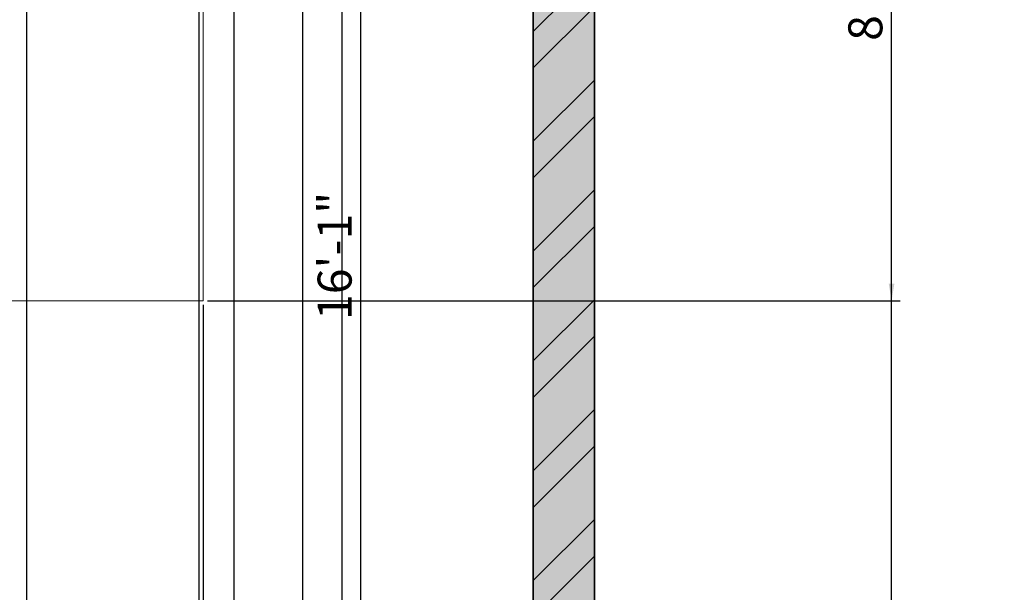
# Model space of a CAD drawing. Units: inches. Extents: x 1804 to 3296, y 909 to 2477.
# Tile 20 of 31: x 2241 to 2386, y 1638 to 1722. Entities that reach past the tile are written whole.
import ezdxf

# ---------------------------------------------------------------- set-up
doc = ezdxf.new("R2010")
doc.units = ezdxf.units.IN
for name, color, linetype, lineweight in [('A-ANNO-DIMS', 2, 'Continuous', 18), ('A-ANNO-TTLB', 156, 'Continuous', 35), ('A-WALL-PATT', 10, 'Continuous', 13), ('FUR', 100, 'Continuous', 18), ('WALL', 10, 'Continuous', 35)]:
    doc.layers.add(name, color=color, linetype=linetype, lineweight=lineweight)
doc.styles.get("Standard").update_dxf_attribs({"font": 'arial.ttf'})
doc.dimstyles.new('ISO-25', dxfattribs={"dimtxt": 5, "dimasz": 2.5, "dimexe": 1.25, "dimexo": 0.625, "dimtad": 1, "dimdec": 0, "dimlunit": 4, "dimtxsty": 'Standard', "dimcen": 2.5, "dimadec": 0, "dimazin": 0, "dimtfac": 1, "dimtdec": 0, "dimtmove": 0, "dimatfit": 3, "dimfxl": 1, "dimarcsym": 0})

# ---------------------------------------------------------------- blocks, each defined once
blk = doc.blocks.new('*D11')
at = {"layer": 'A-ANNO-DIMS', "color": 0, "lineweight": -2, "transparency": 16777216}
for p, q in [((2315.91, 1784.38), (2289.92, 1784.38)), ((2291.17, 1781.88), (2291.17, 1593.42)), ((2315.91, 1590.92), (2289.92, 1590.92))]:
    blk.add_line(p, q, dxfattribs=at)
at = {"layer": 'A-ANNO-DIMS', "color": 0, "lineweight": 100, "transparency": 16777216}
for points in [[(2290.75, 1781.88), (2291.58, 1781.88), (2291.17, 1784.38)], [(2290.75, 1593.42), (2291.58, 1593.42), (2291.17, 1590.92)]]:
    blk.add_solid(points, dxfattribs=at)
at = {"layer": 'Defpoints', "color": 0, "lineweight": 100, "transparency": 16777216}
for p in [(2316.54, 1784.38), (2291.17, 1590.92), (2316.54, 1590.92)]:
    blk.add_point(p, dxfattribs=at)
at = {"layer": 'A-ANNO-DIMS', "color": 0, "transparency": 16777216, "insert": (2287.99, 1687.65), "char_height": 5, "attachment_point": 5, "rotation": 90}
blk.add_mtext('16\'-1"', dxfattribs=at)
blk = doc.blocks.new('*D53')
at = {"layer": 'A-ANNO-DIMS', "color": 0, "lineweight": -2, "transparency": 16777216}
for p, q in [((2326.16, 1793.38), (2370.49, 1793.38)), ((2369.24, 1140.57), (2369.24, 1790.88)), ((2326.16, 1138.07), (2370.49, 1138.07))]:
    blk.add_line(p, q, dxfattribs=at)
at = {"layer": 'A-ANNO-DIMS', "color": 0, "lineweight": 100, "transparency": 16777216}
for points in [[(2368.82, 1790.88), (2369.65, 1790.88), (2369.24, 1793.38)], [(2368.82, 1140.57), (2369.65, 1140.57), (2369.24, 1138.07)]]:
    blk.add_solid(points, dxfattribs=at)
at = {"layer": 'Defpoints', "color": 0, "lineweight": 100, "transparency": 16777216}
for p in [(2325.54, 1793.38), (2369.24, 1793.38), (2325.54, 1138.07)]:
    blk.add_point(p, dxfattribs=at)
at = {"layer": 'A-ANNO-DIMS', "color": 0, "transparency": 16777216, "insert": (2366.03, 1465.72), "char_height": 5, "attachment_point": 5, "rotation": 90}
blk.add_mtext('54\'-7 1/2"', dxfattribs=at)
blk = doc.blocks.new('*D56')
at = {"layer": 'A-ANNO-DIMS', "color": 0, "lineweight": -2, "transparency": 16777216}
for p, q in [((2180.87, 1680.42), (2180.87, 975.89)), ((2268, 1680.42), (2268, 975.89)), ((2183.37, 977.14), (2265.5, 977.14))]:
    blk.add_line(p, q, dxfattribs=at)
at = {"layer": 'A-ANNO-DIMS', "color": 0, "lineweight": 100, "transparency": 16777216}
for points in [[(2183.37, 977.56), (2183.37, 976.72), (2180.87, 977.14)], [(2265.5, 977.56), (2265.5, 976.72), (2268, 977.14)]]:
    blk.add_solid(points, dxfattribs=at)
at = {"layer": 'Defpoints', "color": 0, "lineweight": 100, "transparency": 16777216}
for p in [(2180.87, 1681.04), (2268, 1681.04), (2268, 977.14)]:
    blk.add_point(p, dxfattribs=at)
at = {"layer": 'A-ANNO-DIMS', "color": 0, "transparency": 16777216, "insert": (2224.44, 980.32), "char_height": 5, "attachment_point": 5}
blk.add_mtext('7\'-3"', dxfattribs=at)
blk = doc.blocks.new('*D57')
at = {"layer": 'A-ANNO-DIMS', "color": 0, "lineweight": -2, "transparency": 16777216}
for p, q in [((2268.63, 1784.38), (2370.49, 1784.38)), ((2369.24, 1683.54), (2369.24, 1781.88)), ((2268.63, 1681.04), (2370.49, 1681.04))]:
    blk.add_line(p, q, dxfattribs=at)
at = {"layer": 'A-ANNO-DIMS', "color": 0, "lineweight": 100, "transparency": 16777216}
for points in [[(2368.82, 1781.88), (2369.65, 1781.88), (2369.24, 1784.38)], [(2368.82, 1683.54), (2369.65, 1683.54), (2369.24, 1681.04)]]:
    blk.add_solid(points, dxfattribs=at)
at = {"layer": 'Defpoints', "color": 0, "lineweight": 100, "transparency": 16777216}
for p in [(2268, 1784.38), (2369.24, 1784.38), (2268, 1681.04)]:
    blk.add_point(p, dxfattribs=at)
at = {"layer": 'A-ANNO-DIMS', "color": 0, "transparency": 16777216, "insert": (2366.03, 1732.71), "char_height": 5, "attachment_point": 5, "rotation": 90}
blk.add_mtext('8\'-7 1/2"', dxfattribs=at)
blk = doc.blocks.new('*D65')
at = {"layer": 'A-ANNO-DIMS', "color": 0, "lineweight": -2, "transparency": 16777216}
for p, q in [((2282.65, 1466.57), (2282.65, 1874.99)), ((2316.54, 1466.57), (2316.54, 1874.99)), ((2285.15, 1873.74), (2314.04, 1873.74))]:
    blk.add_line(p, q, dxfattribs=at)
at = {"layer": 'A-ANNO-DIMS', "color": 0, "lineweight": 100, "transparency": 16777216}
for points in [[(2285.15, 1874.15), (2285.15, 1873.32), (2282.65, 1873.74)], [(2314.04, 1874.15), (2314.04, 1873.32), (2316.54, 1873.74)]]:
    blk.add_solid(points, dxfattribs=at)
at = {"layer": 'Defpoints', "color": 0, "lineweight": 100, "transparency": 16777216}
for p in [(2316.54, 1873.74), (2282.65, 1465.94), (2316.54, 1465.94)]:
    blk.add_point(p, dxfattribs=at)
at = {"layer": 'A-ANNO-DIMS', "color": 0, "transparency": 16777216, "insert": (2299.6, 1876.91), "char_height": 5, "attachment_point": 5}
blk.add_mtext('2\'-10"', dxfattribs=at)
blk = doc.blocks.new('*D67')
at = {"layer": 'A-ANNO-DIMS', "color": 0, "lineweight": -2, "transparency": 16777216}
for p, q in [((2267.43, 1587.05), (2267.43, 1874.99)), ((2288.43, 1587.05), (2288.43, 1874.99)), ((2269.93, 1873.74), (2285.93, 1873.74))]:
    blk.add_line(p, q, dxfattribs=at)
at = {"layer": 'A-ANNO-DIMS', "color": 0, "lineweight": 100, "transparency": 16777216}
for points in [[(2269.93, 1874.15), (2269.93, 1873.32), (2267.43, 1873.74)], [(2285.93, 1874.15), (2285.93, 1873.32), (2288.43, 1873.74)]]:
    blk.add_solid(points, dxfattribs=at)
at = {"layer": 'Defpoints', "color": 0, "lineweight": 100, "transparency": 16777216}
for p in [(2288.43, 1873.74), (2267.43, 1586.42), (2288.43, 1586.42)]:
    blk.add_point(p, dxfattribs=at)
at = {"layer": 'A-ANNO-DIMS', "color": 0, "transparency": 16777216, "insert": (2277.93, 1876.91), "char_height": 5, "attachment_point": 5}
blk.add_mtext('1\'-9"', dxfattribs=at)
blk = doc.blocks.new('*D68')
at = {"layer": 'A-ANNO-DIMS', "color": 0, "lineweight": -2, "transparency": 16777216}
for p, q in [((2242.06, 1587.05), (2242.06, 1874.99)), ((2267.43, 1587.05), (2267.43, 1874.99)), ((2244.56, 1873.74), (2264.93, 1873.74)), ((2267.43, 1873.74), (2296.2, 1873.74))]:
    blk.add_line(p, q, dxfattribs=at)
at = {"layer": 'A-ANNO-DIMS', "color": 0, "lineweight": 100, "transparency": 16777216}
for points in [[(2244.56, 1874.15), (2244.56, 1873.32), (2242.06, 1873.74)], [(2264.93, 1874.15), (2264.93, 1873.32), (2267.43, 1873.74)]]:
    blk.add_solid(points, dxfattribs=at)
at = {"layer": 'Defpoints', "color": 0, "lineweight": 100, "transparency": 16777216}
for p in [(2267.43, 1873.74), (2242.06, 1586.42), (2267.43, 1586.42)]:
    blk.add_point(p, dxfattribs=at)
at = {"layer": 'A-ANNO-DIMS', "color": 0, "transparency": 16777216, "insert": (2283.07, 1876.95), "char_height": 5, "attachment_point": 5}
blk.add_mtext('2\'-1 1/2"', dxfattribs=at)
blk = doc.blocks.new('*D73')
at = {"layer": 'A-ANNO-DIMS', "color": 0, "lineweight": -2, "transparency": 16777216}
for p, q in [((2272.59, 1272.26), (2272.59, 1874.99)), ((2316.54, 1272.26), (2316.54, 1874.99)), ((2275.09, 1873.74), (2314.04, 1873.74))]:
    blk.add_line(p, q, dxfattribs=at)
at = {"layer": 'A-ANNO-DIMS', "color": 0, "lineweight": 100, "transparency": 16777216}
for points in [[(2275.09, 1874.15), (2275.09, 1873.32), (2272.59, 1873.74)], [(2314.04, 1874.15), (2314.04, 1873.32), (2316.54, 1873.74)]]:
    blk.add_solid(points, dxfattribs=at)
at = {"layer": 'Defpoints', "color": 0, "lineweight": 100, "transparency": 16777216}
for p in [(2316.54, 1873.74), (2272.59, 1271.63), (2316.54, 1271.63)]:
    blk.add_point(p, dxfattribs=at)
at = {"layer": 'A-ANNO-DIMS', "color": 0, "transparency": 16777216, "insert": (2294.56, 1876.92), "char_height": 5, "attachment_point": 5}
blk.add_mtext('3\'-8"', dxfattribs=at)

msp = doc.modelspace()

# ---------------------------------------------------------------- hatches: boundary and pattern name
at = {"layer": 'A-ANNO-TTLB'}
h = msp.add_hatch(color=256, dxfattribs=at)
h.dxf.hatch_style = 1
h.paths.add_polyline_path([(3294.53, 2476.54), (1803.79, 2476.54), (1805.43, 909.47), (3296.17, 909.47)])
h.paths.add_polyline_path([(1811, 914.33), (1812.79, 2467.54), (3285.53, 2467.54), (3283.74, 914.33)], flags=16)
h.paths.add_polyline_path([(1925.58, 1062.77), (1925.58, 1138.07), (1925.58, 1539.88), (1925.58, 1793.38), (1925.58, 1830.04), (2325.54, 1830.04), (2325.54, 1793.38), (2325.54, 1586.42), (2325.54, 1138.07), (2325.54, 1062.77)], flags=0)
h.paths.add_polyline_path([(1997.22, 1029.4), (2008.85, 1037.96), (2008.85, 1020.84)], flags=0)
h.paths.add_polyline_path([(1934.58, 1138.07), (1934.58, 1147.07), (2078.77, 1147.07), (2078.77, 1138.07), (2060.94, 1138.07)], flags=0)
h.paths.add_polyline_path([(1944.35, 1138.07), (1944.35, 1147.07), (2056.05, 1147.07), (2056.05, 1138.07)], flags=0)
h.paths.add_polyline_path([(2222.24, 1037.96), (2233.87, 1029.4), (2222.24, 1020.84)], flags=0)
h.paths.add_polyline_path([(2061.94, 1139.07), (2061.94, 1146.07), (2077.77, 1146.07), (2077.77, 1139.07)], flags=0)
h.paths.add_polyline_path([(2149.58, 1138.07), (2149.58, 1269.44), (2158.58, 1269.44), (2158.58, 1326.69), (2149.58, 1326.69), (2149.58, 1340.94), (2139.6, 1340.94), (2139.6, 1434.25), (2149.58, 1434.25), (2149.58, 1447.36), (2158.58, 1447.36), (2158.58, 1423.87), (2158.58, 1408.06), (2198.46, 1408.06), (2198.46, 1412.56), (2282.65, 1412.56), (2282.65, 1465.94), (2316.54, 1465.94), (2316.54, 1590.92), (2192.86, 1590.92), (2192.86, 1595.3), (2291.17, 1595.3), (2291.17, 1590.92), (2316.54, 1590.92), (2316.54, 1784.38), (2300.24, 1784.38), (2300.24, 1757.47), (2268, 1757.47), (2268, 1681.04), (2180.87, 1681.04), (2180.87, 1757.47), (2148.63, 1757.47), (2148.63, 1784.38), (2119.08, 1784.38), (2119.08, 1585.58), (2114.58, 1585.58), (2114.58, 1784.38), (2064.11, 1784.38), (2046.28, 1784.38), (2046.28, 1760.38), (1958.58, 1760.38), (1958.58, 1664.38), (1934.58, 1664.38), (1934.58, 1784.38), (1934.58, 1793.38), (2046.28, 1793.38), (2064.11, 1793.38), (2119.08, 1793.38), (2230.78, 1793.38), (2230.78, 1784.38), (2268, 1784.38), (2300.24, 1784.38), (2316.54, 1784.38), (2316.54, 1590.92), (2316.54, 1373.73), (2316.54, 1138.07)], flags=0)
h.paths.add_polyline_path([(2209.19, 1166.63), (2209.19, 1175.63), (2158.58, 1175.63), (2209.19, 1223.63), (2209.19, 1231.63), (2183.88, 1231.63), (2183.88, 1301.66), (2242.59, 1301.66), (2242.59, 1326.69), (2316.54, 1326.69), (2272.59, 1271.63), (2272.59, 1223.63), (2316.54, 1175.63), (2272.59, 1175.63), (2272.59, 1166.63)], flags=0)
h.paths.add_polyline_path([(1947.77, 1345.22), (1947.77, 1457.48), (1991.2, 1457.48), (1991.2, 1451.7), (1991.2, 1352.18), (1991.2, 1345.22)], flags=0)
h.paths.add_polyline_path([(2209.19, 1271.63), (2262.59, 1271.63), (2262.59, 1311.85), (2272.59, 1301.66), (2272.59, 1271.63), (2269.92, 1269.63), (2270.59, 1269.63), (2270.59, 1225.63), (2211.19, 1225.63), (2211.19, 1269.63), (2211.86, 1269.63)], flags=0)
h.paths.add_polyline_path([(2000.34, 1378.21), (2000.34, 1429.71), (2025.22, 1429.71), (2025.22, 1378.21)], flags=0)
h.paths.add_polyline_path([(2001.34, 1379.21), (2001.34, 1428.71), (2024.22, 1428.71), (2024.22, 1379.21)], flags=0)
h.paths.add_polyline_path([(2012.34, 1390.21), (2012.34, 1417.71), (2013.22, 1417.71), (2013.22, 1390.21)], flags=0)
h.paths.add_polyline_path([(2237.56, 1331.19), (2237.56, 1340.18), (2238.62, 1340.18), (2238.62, 1386.84), (2241.04, 1386.84), (2242.06, 1386.84), (2242.06, 1408.06), (2316.54, 1331.19)], flags=0)
h.paths.add_polyline_path([(1953.73, 1464.35), (1953.73, 1498.59), (1981.74, 1498.59), (1981.74, 1464.35)], flags=0)
h.paths.add_polyline_path([(1987.63, 1462.08), (1987.63, 1500.95), (2104.07, 1500.95), (2104.07, 1462.08), (2099.27, 1462.08), (1993.6, 1462.08)], flags=0)
h.paths.add_polyline_path([(1956.06, 1481.47, -1), (1979.41, 1481.47, -1)], flags=0)
edge = h.paths.add_edge_path(flags=0)
edge.add_ellipse((2299.53, 1438.37), major_axis=(0.31, 21.36), ratio=0.670333, start_angle=0, end_angle=360)
h.paths.add_polyline_path([(2297.39, 1438.37, -1), (2301.67, 1438.37, -1)], flags=0)
h.paths.add_polyline_path([(2591.54, 1163.23), (2591.54, 1179.38), (2591.54, 1379.68), (2591.54, 1395.84), (2734.5, 1395.84), (2734.5, 1379.68), (2734.5, 1179.38), (2734.5, 1163.23)], flags=0)
h.paths.add_polyline_path([(2592.54, 1164.23), (2592.54, 1166.23), (2733.5, 1166.23), (2733.5, 1164.23)], flags=0)
h.paths.add_polyline_path([(2592.54, 1180.38), (2592.54, 1378.68), (2733.5, 1378.68), (2733.5, 1180.38)], flags=0)
h.paths.add_polyline_path([(2593.54, 1181.38), (2593.54, 1377.68), (2732.5, 1377.68), (2732.5, 1181.38)], flags=0)
h.paths.add_polyline_path([(2594.54, 1182.38), (2594.54, 1376.68), (2731.5, 1376.68), (2731.5, 1182.38)], flags=0)
h.paths.add_polyline_path([(1936.95, 1697.46), (1936.95, 1736.46), (1955.41, 1736.46), (1955.41, 1697.46)], flags=0)
h.paths.add_polyline_path([(1938.48, 1718.36), (1938.48, 1734.92), (1953.65, 1734.92), (1953.65, 1718.36)], flags=0)
h.paths.add_polyline_path([(1944.75, 1726.64, -1), (1947.37, 1726.64, -1)], flags=0)
h.paths.add_polyline_path([(2592.54, 1394.84), (2733.5, 1394.84), (2733.5, 1392.84), (2592.54, 1392.84)], flags=0)
h.paths.add_polyline_path([(1976.61, 1762.5), (1976.61, 1781.44), (2012.79, 1781.44), (2012.79, 1762.5)], flags=0)
h.paths.add_polyline_path([(1979.57, 1771.97, -1), (1991.39, 1771.97, -1)], flags=0)
h.paths.add_polyline_path([(1995.36, 1771.97, -1), (2007.18, 1771.97, -1)], flags=0)
h.paths.add_polyline_path([(2251.51, 1744.53), (2268, 1730.05), (2251.51, 1730.05)], flags=0)
h.paths.add_polyline_path([(2047.28, 1785.38), (2047.28, 1792.38), (2063.11, 1792.38), (2063.11, 1785.38)], flags=0)
h.paths.add_polyline_path([(2155.08, 1770.92, -1), (2174.42, 1770.92, -1)], flags=0)
h.paths.add_polyline_path([(2188.59, 1758.27), (2188.59, 1772.81), (2222.3, 1772.81), (2222.3, 1758.27)], flags=0)
h.paths.add_polyline_path([(2223.97, 1758.27), (2223.97, 1772.81), (2257.68, 1772.81), (2257.68, 1758.27)], flags=0)
h.paths.add_polyline_path([(2274.45, 1770.92, -1), (2293.8, 1770.92, -1)], flags=0)
h.paths.add_polyline_path([(2591.54, 1582.09), (2591.54, 1782.39), (2734.5, 1782.39), (2734.5, 1582.09)], flags=0)
h.paths.add_polyline_path([(2592.54, 1583.09), (2592.54, 1781.39), (2733.5, 1781.39), (2733.5, 1583.09)], flags=0)
h.paths.add_polyline_path([(2593.54, 1584.09), (2593.54, 1780.39), (2732.5, 1780.39), (2732.5, 1584.09)], flags=0)
h.paths.add_polyline_path([(2594.54, 1585.09), (2594.54, 1779.39), (2731.5, 1779.39), (2731.5, 1585.09)], flags=0)
h.paths.add_polyline_path([(1922.17, 1978.79), (1922.17, 2295.08), (1922.17, 2296.08), (2115.67, 2296.08), (2115.67, 2384.31), (2115.67, 2385.31), (2322.12, 2385.31), (2323.12, 2385.31), (2323.12, 1979.79), (2323.12, 1978.79), (1923.17, 1978.79)], flags=0)
h.paths.add_polyline_path([(1922.17, 1978.79), (1922.17, 2051.31), (1922.17, 2214.86), (1922.17, 2296.08), (2115.67, 2296.08), (2115.67, 2385.31), (2323.12, 2385.31), (2323.12, 2280.42), (2323.12, 1978.79), (2115.67, 1978.79)], flags=0)
h.paths.add_polyline_path([(1923.17, 1979.79), (1923.17, 2050.31), (2115.67, 2050.31), (2115.67, 2051.31), (1923.17, 2051.31), (1923.17, 2213.86), (1923.17, 2214.86), (1923.17, 2295.08), (1990.02, 2295.08), (1990.02, 2214.86), (1991.02, 2214.86), (1991.02, 2295.08), (2115.67, 2295.08), (2115.67, 1979.79), (2116.67, 1979.79), (2116.67, 2304.18), (2116.67, 2384.31), (2322.12, 2384.31), (2322.12, 2280.42), (2322.12, 1979.79), (2115.67, 1979.79)], flags=0)
h.paths.add_polyline_path([(2972.46, 1192.5), (2972.46, 1196.92), (2995.47, 1196.92), (2995.47, 1255.47), (2995.09, 1255.47), (2987.42, 1249.39), (2980.08, 1255.47), (2978.05, 1255.47), (2978.05, 1257.24), (2995.47, 1257.24), (2995.47, 1261.58), (3015.37, 1261.58), (3015.37, 1333.28), (3015.37, 1414.4), (3032.82, 1414.4), (3032.82, 1333.28), (3032.82, 1261.58), (3052.66, 1261.58), (3052.66, 1255.47), (3079.86, 1255.47), (3078.72, 1254.57), (3081.47, 1252.29), (3078.56, 1249.99), (3075.81, 1252.26), (3072.57, 1249.69), (3070.36, 1251.52), (3067.67, 1249.39), (3060.34, 1255.47), (3052.66, 1255.47), (3052.66, 1196.92), (3054.58, 1196.92), (3074, 1196.92), (3074, 1192.5), (3052.66, 1192.5), (2995.47, 1192.5)], flags=0)
h.paths.add_polyline_path([(2490.75, 1979.27), (2490.75, 1980.27), (2596.87, 1980.27), (2596.87, 2051.8), (2596.87, 2052.8), (2596.87, 2216.35), (2596.87, 2297.57), (2717.32, 2297.57), (2710.57, 2305.62), (2724.07, 2305.62), (2717.32, 2297.57), (2782.37, 2297.57), (2782.37, 2395.8), (3006.82, 2395.8), (3006.82, 1981.27), (3093.73, 1981.27), (3093.73, 1980.27), (3047.51, 1980.27), (3046.37, 1979.37), (3049.11, 1977.1), (3046.2, 1974.79), (3043.46, 1977.07), (3040.21, 1974.49), (3038, 1976.32), (3035.32, 1974.2), (3027.98, 1980.27), (2871.83, 1980.27), (2871.83, 1981.27), (2791.37, 1981.27), (2791.37, 2050.8), (2597.87, 2050.8), (2597.87, 1980.27), (2597.87, 1979.27), (2546.27, 1979.27), (2545.12, 1978.37), (2547.87, 1976.1), (2544.96, 1973.79), (2542.22, 1976.07), (2538.97, 1973.49), (2536.76, 1975.32), (2534.07, 1973.2), (2526.74, 1979.27)], flags=0)
h.paths.add_polyline_path([(2597.87, 2051.8), (2606.87, 2051.8), (2606.87, 2258.39), (2597.87, 2258.39), (2597.87, 2296.57), (2606.87, 2296.57), (2606.87, 2262.39), (2782.37, 2262.39), (2782.37, 2296.57), (2790.37, 2296.57), (2790.37, 2262.39), (2791.37, 2262.39), (2791.37, 2305.67), (2791.37, 2385.8), (2996.82, 2385.8), (2996.82, 2339.85), (3006.82, 2339.85), (3006.82, 2250.12), (2997.82, 2250.12), (2997.82, 1981.27), (2996.82, 1981.27), (2872.83, 1981.27), (2872.83, 1991.8), (2871.83, 1991.8), (2871.83, 2050.8), (2790.37, 2050.8), (2597.87, 2050.8)], flags=0)
h.paths.add_polyline_path([(2179.93, 2153.92), (2179.93, 2353.97), (2259.98, 2353.97), (2259.98, 2153.92)], flags=0)
h.paths.add_polyline_path([(2180.93, 2154.92), (2180.93, 2352.97), (2258.98, 2352.97), (2258.98, 2154.92)], flags=0)
h.paths.add_polyline_path([(2960.87, 1608.49), (2960.87, 1753.62), (3070.9, 1753.62), (3070.9, 1608.49)], flags=0)
h.paths.add_polyline_path([(2961.87, 1609.49), (2961.87, 1752.62), (3069.9, 1752.62), (3069.9, 1609.49)], flags=0)
h.paths.add_polyline_path([(2962.87, 1610.49), (2962.87, 1751.62), (3068.9, 1751.62), (3068.9, 1610.49)], flags=0)
h.paths.add_polyline_path([(2963.87, 1611.49), (2963.87, 1750.62), (3067.9, 1750.62), (3067.9, 1611.49)], flags=0)
h.paths.add_polyline_path([(2782.37, 2051.8), (2782.37, 2216.32), (2791.37, 2216.32), (2791.37, 2051.8), (2872.83, 2051.8), (2872.83, 2068.56), (2884.67, 2068.56), (2884.67, 2085.33), (2896.51, 2085.33), (2896.51, 2102.09), (2908.36, 2102.09), (2908.36, 2118.85), (2920.2, 2118.85), (2920.2, 2135.62), (2932.05, 2135.62), (2932.05, 2145.3), (2925.08, 2145.3), (2925.08, 2203.2), (2996.82, 2203.2), (2996.82, 2145.3), (2953.82, 2145.3), (2872.83, 2051.8), (2790.37, 2051.8)], flags=0)
h.paths.add_polyline_path([(2717.32, 2238.65), (2710.57, 2246.7), (2724.07, 2246.7)], flags=0)
h.paths.add_polyline_path([(2003.09, 1122.79), (2017.16, 1122.79), (2017.16, 1138.74), (2003.09, 1138.74)], flags=8)
h.paths.add_polyline_path([(2174.76, 1792.72), (2188.83, 1792.72), (2188.83, 1808.66), (2174.76, 1808.66)], flags=8)
h.paths.add_polyline_path([(1987.95, 1792.51), (2002.02, 1792.51), (2002.02, 1808.45), (1987.95, 1808.45)], flags=8)
h.paths.add_polyline_path([(2148.79, 1289.26), (2160.46, 1289.26), (2160.46, 1305.2), (2148.79, 1305.2)], flags=8)
h.paths.add_polyline_path([(2115.36, 1133.57), (2127.04, 1133.57), (2127.04, 1149.51), (2115.36, 1149.51)], flags=8)
h.paths.add_polyline_path([(2237.58, 1421.48), (2249.25, 1421.48), (2249.25, 1437.43), (2237.58, 1437.43)], flags=8)
h.paths.add_polyline_path([(2134.99, 1584.32), (2146.66, 1584.32), (2146.66, 1600.26), (2134.99, 1600.26)], flags=8)
h.paths.add_polyline_path([(2101.95, 1557.31), (2113.62, 1557.31), (2113.62, 1573.25), (2101.95, 1573.25)], flags=8)
h.paths.add_polyline_path([(2937.85, 1156.77), (3120.41, 1156.77), (3120.41, 1185.72), (2937.85, 1185.72)], flags=8)
h.paths.add_polyline_path([(2980.71, 1786.71), (3050.06, 1786.71), (3050.06, 1802.66), (2980.71, 1802.66)], flags=8)
h.paths.add_polyline_path([(2869.28, 1661.96), (2938.62, 1661.96), (2938.62, 1690.8), (2869.28, 1690.8)], flags=8)
h.paths.add_polyline_path([(3092.27, 1674.86), (3161.62, 1674.86), (3161.62, 1690.8), (3092.27, 1690.8)], flags=8)
h.paths.add_polyline_path([(2980.71, 1674.86), (3050.06, 1674.86), (3050.06, 1690.8), (2980.71, 1690.8)], flags=8)
h.paths.add_polyline_path([(2649.07, 1678.23), (2674.53, 1678.23), (2674.53, 1714.76), (2649.07, 1714.76)], flags=8)
h.paths.add_polyline_path([(2530.84, 1981.63), (2549.13, 1981.63), (2549.13, 1997.57), (2530.84, 1997.57)], flags=8)
h.paths.add_polyline_path([(3031.29, 1981.77), (3049.58, 1981.77), (3049.58, 1997.71), (3031.29, 1997.71)], flags=8)
h.paths.add_polyline_path([(2715.38, 1911.9), (2851.54, 1911.9), (2851.54, 1940.85), (2715.38, 1940.85)], flags=8)
h.paths.add_polyline_path([(2015.23, 1927.36), (2205.42, 1927.36), (2205.42, 1956.3), (2015.23, 1956.3)], flags=8)
h.paths.add_polyline_path([(2671.84, 2057.84), (2702.75, 2057.84), (2702.75, 2073.79), (2671.84, 2073.79)], flags=8)
h.paths.add_polyline_path([(2678.5, 2316.52), (2765.26, 2316.52), (2765.26, 2332.46), (2678.5, 2332.46)], flags=8)
h.paths.add_polyline_path([(2678.48, 2271.96), (2736.41, 2271.96), (2736.41, 2287.9), (2678.48, 2287.9)], flags=8)
h.paths.add_polyline_path([(2019.2, 972.79), (2243.21, 972.79), (2243.21, 1001.74), (2019.2, 1001.74)], flags=8)
h.paths.add_polyline_path([(2097.06, 1021.56), (2132.16, 1021.56), (2132.16, 1037.51), (2097.06, 1037.51)], flags=8)
h.paths.add_polyline_path([(2182.47, 1360.48), (2207.35, 1360.48), (2207.35, 1376.42), (2182.47, 1376.42)], flags=8)
h.paths.add_polyline_path([(2261.12, 1361.77), (2295.01, 1361.77), (2295.01, 1377.71), (2261.12, 1377.71)], flags=8)
h.paths.add_polyline_path([(2245.75, 1511.51), (2278.44, 1511.51), (2278.44, 1527.46), (2245.75, 1527.46)], flags=8)
h.paths.add_polyline_path([(1991.16, 1296.29), (2060.51, 1296.29), (2060.51, 1312.23), (1991.16, 1312.23)], flags=8)
h.paths.add_polyline_path([(2187, 1651.35), (2246.71, 1651.35), (2246.71, 1667.29), (2187, 1667.29)], flags=8)
h.paths.add_polyline_path([(1976.49, 1684.81), (2068.63, 1684.81), (2068.63, 1700.76), (1976.49, 1700.76)], flags=8)
at = {"layer": 'A-WALL-PATT'}
h = msp.add_hatch(color=256, dxfattribs=at)
h.dxf.hatch_style = 1
h.paths.add_polyline_path([(2119.08, 1544.38), (1925.58, 1544.38), (1925.58, 1539.88), (2119.08, 1539.88)])
h.paths.add_polyline_path([(2119.08, 1545.58), (2114.58, 1545.58), (2114.58, 1544.38), (2119.08, 1544.38)])
h.paths.add_polyline_path([(1965.87, 1658.79), (1965.87, 1679.09), (1955.57, 1679.09), (1955.57, 1658.79)], flags=9)
h.paths.add_polyline_path([(2293.18, 1677.29), (2293.18, 1697.58), (2282.88, 1697.58), (2282.88, 1677.29)], flags=9)
h.paths.add_polyline_path([(2271.13, 1545.23), (2287.53, 1545.23), (2287.53, 1555.53), (2271.13, 1555.53)], flags=9)
h.paths.add_polyline_path([(2303.26, 1488.52), (2303.26, 1508.82), (2292.95, 1508.82), (2292.95, 1488.52)], flags=9)
h.paths.add_polyline_path([(2271.13, 1393.15), (2287.53, 1393.15), (2287.53, 1403.45), (2271.13, 1403.45)], flags=9)
h.paths.add_polyline_path([(2306.48, 1361.45), (2306.48, 1377.86), (2296.18, 1377.86), (2296.18, 1361.45)], flags=9)
h.paths.add_polyline_path([(2174.54, 1361.45), (2174.54, 1377.86), (2164.23, 1377.86), (2164.23, 1361.45)], flags=9)
h.paths.add_polyline_path([(1968.21, 1333.34), (1968.21, 1353.64), (1957.91, 1353.64), (1957.91, 1333.34)], flags=9)
h.paths.add_polyline_path([(2003.09, 1122.79), (2017.16, 1122.79), (2017.16, 1138.74), (2003.09, 1138.74)], flags=9)
h.paths.add_polyline_path([(2174.76, 1792.72), (2188.83, 1792.72), (2188.83, 1808.66), (2174.76, 1808.66)], flags=9)
h.paths.add_polyline_path([(1987.95, 1792.51), (2002.02, 1792.51), (2002.02, 1808.45), (1987.95, 1808.45)], flags=9)
h.paths.add_polyline_path([(2148.79, 1289.26), (2160.46, 1289.26), (2160.46, 1305.2), (2148.79, 1305.2)], flags=9)
h.paths.add_polyline_path([(2115.36, 1133.57), (2127.04, 1133.57), (2127.04, 1149.51), (2115.36, 1149.51)], flags=9)
h.paths.add_polyline_path([(2237.58, 1421.48), (2249.25, 1421.48), (2249.25, 1437.43), (2237.58, 1437.43)], flags=9)
h.paths.add_polyline_path([(2134.99, 1584.32), (2146.66, 1584.32), (2146.66, 1600.26), (2134.99, 1600.26)], flags=9)
h.paths.add_polyline_path([(2101.95, 1557.31), (2113.62, 1557.31), (2113.62, 1573.25), (2101.95, 1573.25)], flags=9)
h.paths.add_polyline_path([(2937.85, 1156.77), (3120.41, 1156.77), (3120.41, 1185.72), (2937.85, 1185.72)], flags=9)
h.paths.add_polyline_path([(2980.71, 1786.71), (3050.06, 1786.71), (3050.06, 1802.66), (2980.71, 1802.66)], flags=9)
h.paths.add_polyline_path([(2869.28, 1661.96), (2938.62, 1661.96), (2938.62, 1690.8), (2869.28, 1690.8)], flags=9)
h.paths.add_polyline_path([(3092.27, 1674.86), (3161.62, 1674.86), (3161.62, 1690.8), (3092.27, 1690.8)], flags=9)
h.paths.add_polyline_path([(2980.71, 1674.86), (3050.06, 1674.86), (3050.06, 1690.8), (2980.71, 1690.8)], flags=9)
h.paths.add_polyline_path([(2649.07, 1678.23), (2674.53, 1678.23), (2674.53, 1714.76), (2649.07, 1714.76)], flags=9)
h.paths.add_polyline_path([(2530.84, 1981.63), (2549.13, 1981.63), (2549.13, 1997.57), (2530.84, 1997.57)], flags=9)
h.paths.add_polyline_path([(3031.29, 1981.77), (3049.58, 1981.77), (3049.58, 1997.71), (3031.29, 1997.71)], flags=9)
h.paths.add_polyline_path([(2715.38, 1911.9), (2851.54, 1911.9), (2851.54, 1940.85), (2715.38, 1940.85)], flags=9)
h.paths.add_polyline_path([(2015.23, 1927.36), (2205.42, 1927.36), (2205.42, 1956.3), (2015.23, 1956.3)], flags=9)
h.paths.add_polyline_path([(2671.84, 2057.84), (2702.75, 2057.84), (2702.75, 2073.79), (2671.84, 2073.79)], flags=9)
h.paths.add_polyline_path([(2678.5, 2316.52), (2765.26, 2316.52), (2765.26, 2332.46), (2678.5, 2332.46)], flags=9)
h.paths.add_polyline_path([(2678.48, 2271.96), (2736.41, 2271.96), (2736.41, 2287.9), (2678.48, 2287.9)], flags=9)
h.paths.add_polyline_path([(2019.2, 972.79), (2243.21, 972.79), (2243.21, 1001.74), (2019.2, 1001.74)], flags=9)
h.paths.add_polyline_path([(2097.06, 1021.56), (2132.16, 1021.56), (2132.16, 1037.51), (2097.06, 1037.51)], flags=9)
h.paths.add_polyline_path([(2182.47, 1360.48), (2207.35, 1360.48), (2207.35, 1376.42), (2182.47, 1376.42)], flags=9)
h.paths.add_polyline_path([(2261.12, 1361.77), (2295.01, 1361.77), (2295.01, 1377.71), (2261.12, 1377.71)], flags=9)
h.paths.add_polyline_path([(2245.75, 1511.51), (2278.44, 1511.51), (2278.44, 1527.46), (2245.75, 1527.46)], flags=9)
h.paths.add_polyline_path([(1991.16, 1296.29), (2060.51, 1296.29), (2060.51, 1312.23), (1991.16, 1312.23)], flags=9)
h.paths.add_polyline_path([(2187, 1651.35), (2246.71, 1651.35), (2246.71, 1667.29), (2187, 1667.29)], flags=9)
h.paths.add_polyline_path([(1976.49, 1684.81), (2068.63, 1684.81), (2068.63, 1700.76), (1976.49, 1700.76)], flags=9)
h = msp.add_hatch(color=256, dxfattribs=at)
h.dxf.hatch_style = 1
h.paths.add_polyline_path([(2149.58, 1147.07), (2141.21, 1147.07), (2141.21, 1144.07), (2141.21, 1138.07), (2149.58, 1138.07)])
h.paths.add_polyline_path([(2101.21, 1144.07, -0.01877), (2101.32, 1147.07), (2078.77, 1147.07), (2078.77, 1138.07), (2101.21, 1138.07)])
h.paths.add_polyline_path([(2060.94, 1147.07), (2056.05, 1147.07), (2056.05, 1138.07), (2060.94, 1138.07)])
h.paths.add_polyline_path([(1944.35, 1147.07), (1934.58, 1147.07), (1934.58, 1138.07), (1944.35, 1138.07)])
h.paths.add_polyline_path([(2158.58, 1269.44), (2149.58, 1269.44), (2149.58, 1138.07), (2158.58, 1138.07)])
h.paths.add_polyline_path([(2003.09, 1122.79), (2017.16, 1122.79), (2017.16, 1138.74), (2003.09, 1138.74)], flags=9)
h.paths.add_polyline_path([(2174.76, 1792.72), (2188.83, 1792.72), (2188.83, 1808.66), (2174.76, 1808.66)], flags=9)
h.paths.add_polyline_path([(1987.95, 1792.51), (2002.02, 1792.51), (2002.02, 1808.45), (1987.95, 1808.45)], flags=9)
h.paths.add_polyline_path([(2148.79, 1289.26), (2160.46, 1289.26), (2160.46, 1305.2), (2148.79, 1305.2)], flags=9)
h.paths.add_polyline_path([(2115.36, 1133.57), (2127.04, 1133.57), (2127.04, 1149.51), (2115.36, 1149.51)], flags=9)
h.paths.add_polyline_path([(2237.58, 1421.48), (2249.25, 1421.48), (2249.25, 1437.43), (2237.58, 1437.43)], flags=9)
h.paths.add_polyline_path([(2134.99, 1584.32), (2146.66, 1584.32), (2146.66, 1600.26), (2134.99, 1600.26)], flags=9)
h.paths.add_polyline_path([(2101.95, 1557.31), (2113.62, 1557.31), (2113.62, 1573.25), (2101.95, 1573.25)], flags=9)
h.paths.add_polyline_path([(2937.85, 1156.77), (3120.41, 1156.77), (3120.41, 1185.72), (2937.85, 1185.72)], flags=9)
h.paths.add_polyline_path([(2980.71, 1786.71), (3050.06, 1786.71), (3050.06, 1802.66), (2980.71, 1802.66)], flags=9)
h.paths.add_polyline_path([(2869.28, 1661.96), (2938.62, 1661.96), (2938.62, 1690.8), (2869.28, 1690.8)], flags=9)
h.paths.add_polyline_path([(3092.27, 1674.86), (3161.62, 1674.86), (3161.62, 1690.8), (3092.27, 1690.8)], flags=9)
h.paths.add_polyline_path([(2980.71, 1674.86), (3050.06, 1674.86), (3050.06, 1690.8), (2980.71, 1690.8)], flags=9)
h.paths.add_polyline_path([(2649.07, 1678.23), (2674.53, 1678.23), (2674.53, 1714.76), (2649.07, 1714.76)], flags=9)
h.paths.add_polyline_path([(2530.84, 1981.63), (2549.13, 1981.63), (2549.13, 1997.57), (2530.84, 1997.57)], flags=9)
h.paths.add_polyline_path([(3031.29, 1981.77), (3049.58, 1981.77), (3049.58, 1997.71), (3031.29, 1997.71)], flags=9)
h.paths.add_polyline_path([(2715.38, 1911.9), (2851.54, 1911.9), (2851.54, 1940.85), (2715.38, 1940.85)], flags=9)
h.paths.add_polyline_path([(2015.23, 1927.36), (2205.42, 1927.36), (2205.42, 1956.3), (2015.23, 1956.3)], flags=9)
h.paths.add_polyline_path([(2671.84, 2057.84), (2702.75, 2057.84), (2702.75, 2073.79), (2671.84, 2073.79)], flags=9)
h.paths.add_polyline_path([(2678.5, 2316.52), (2765.26, 2316.52), (2765.26, 2332.46), (2678.5, 2332.46)], flags=9)
h.paths.add_polyline_path([(2678.48, 2271.96), (2736.41, 2271.96), (2736.41, 2287.9), (2678.48, 2287.9)], flags=9)
h.paths.add_polyline_path([(2019.2, 972.79), (2243.21, 972.79), (2243.21, 1001.74), (2019.2, 1001.74)], flags=9)
h.paths.add_polyline_path([(2097.06, 1021.56), (2132.16, 1021.56), (2132.16, 1037.51), (2097.06, 1037.51)], flags=9)
h.paths.add_polyline_path([(2182.47, 1360.48), (2207.35, 1360.48), (2207.35, 1376.42), (2182.47, 1376.42)], flags=9)
h.paths.add_polyline_path([(2261.12, 1361.77), (2295.01, 1361.77), (2295.01, 1377.71), (2261.12, 1377.71)], flags=9)
h.paths.add_polyline_path([(2245.75, 1511.51), (2278.44, 1511.51), (2278.44, 1527.46), (2245.75, 1527.46)], flags=9)
h.paths.add_polyline_path([(1991.16, 1296.29), (2060.51, 1296.29), (2060.51, 1312.23), (1991.16, 1312.23)], flags=9)
h.paths.add_polyline_path([(2187, 1651.35), (2246.71, 1651.35), (2246.71, 1667.29), (2187, 1667.29)], flags=9)
h.paths.add_polyline_path([(1976.49, 1684.81), (2068.63, 1684.81), (2068.63, 1700.76), (1976.49, 1700.76)], flags=9)
h = msp.add_hatch(color=256, dxfattribs=at)
h.dxf.hatch_style = 1
h.paths.add_polyline_path([(2158.58, 1275.49), (2155.29, 1275.49), (2149.58, 1275.49), (2149.58, 1269.44), (2158.58, 1269.44)])
h.paths.add_polyline_path([(2158.58, 1326.69), (2149.58, 1326.69), (2149.58, 1319.33), (2155.29, 1319.33), (2158.58, 1319.33)])
h.paths.add_polyline_path([(2158.58, 1402.2), (2158.58, 1423.87), (2158.58, 1447.36), (2149.58, 1447.36), (2149.58, 1423.87), (2149.58, 1340.94), (2149.58, 1326.69), (2158.58, 1326.69), (2158.58, 1354.23)])
h.paths.add_polyline_path([(1965.87, 1658.79), (1965.87, 1679.09), (1955.57, 1679.09), (1955.57, 1658.79)], flags=9)
h.paths.add_polyline_path([(2293.18, 1677.29), (2293.18, 1697.58), (2282.88, 1697.58), (2282.88, 1677.29)], flags=9)
h.paths.add_polyline_path([(2271.13, 1545.23), (2287.53, 1545.23), (2287.53, 1555.53), (2271.13, 1555.53)], flags=9)
h.paths.add_polyline_path([(2303.26, 1488.52), (2303.26, 1508.82), (2292.95, 1508.82), (2292.95, 1488.52)], flags=9)
h.paths.add_polyline_path([(2271.13, 1393.15), (2287.53, 1393.15), (2287.53, 1403.45), (2271.13, 1403.45)], flags=9)
h.paths.add_polyline_path([(2306.48, 1361.45), (2306.48, 1377.86), (2296.18, 1377.86), (2296.18, 1361.45)], flags=9)
h.paths.add_polyline_path([(2189.9, 1340.62), (2206.31, 1340.62), (2206.31, 1350.92), (2189.9, 1350.92)], flags=9)
h.paths.add_polyline_path([(2174.54, 1361.45), (2174.54, 1377.86), (2164.23, 1377.86), (2164.23, 1361.45)], flags=9)
h.paths.add_polyline_path([(2304.24, 1240.8), (2304.24, 1261.09), (2293.94, 1261.09), (2293.94, 1240.8)], flags=9)
h.paths.add_polyline_path([(2227.19, 1188.73), (2247.49, 1188.73), (2247.49, 1199.03), (2227.19, 1199.03)], flags=9)
h.paths.add_polyline_path([(2181.93, 1144.21), (2181.93, 1160.62), (2171.63, 1160.62), (2171.63, 1144.21)], flags=9)
h.paths.add_polyline_path([(1968.21, 1333.34), (1968.21, 1353.64), (1957.91, 1353.64), (1957.91, 1333.34)], flags=9)
h.paths.add_polyline_path([(2029.78, 1203.53), (2053.95, 1203.53), (2053.95, 1213.83), (2029.78, 1213.83)], flags=9)
h.paths.add_polyline_path([(2576.51, 1671.88), (2576.51, 1692.17), (2566.21, 1692.17), (2566.21, 1671.88)], flags=9)
h.paths.add_polyline_path([(2566.99, 1269.67), (2566.99, 1289.96), (2556.68, 1289.96), (2556.68, 1269.67)], flags=9)
h.paths.add_polyline_path([(2581.85, 1269.17), (2581.85, 1289.46), (2571.54, 1289.46), (2571.54, 1269.17)], flags=9)
h.paths.add_polyline_path([(2650.71, 1409.75), (2674.89, 1409.75), (2674.89, 1420.05), (2650.71, 1420.05)], flags=9)
h.paths.add_polyline_path([(2003.09, 1122.79), (2017.16, 1122.79), (2017.16, 1138.74), (2003.09, 1138.74)], flags=9)
h.paths.add_polyline_path([(2174.76, 1792.72), (2188.83, 1792.72), (2188.83, 1808.66), (2174.76, 1808.66)], flags=9)
h.paths.add_polyline_path([(1987.95, 1792.51), (2002.02, 1792.51), (2002.02, 1808.45), (1987.95, 1808.45)], flags=9)
h.paths.add_polyline_path([(2148.79, 1289.26), (2160.46, 1289.26), (2160.46, 1305.2), (2148.79, 1305.2)], flags=9)
h.paths.add_polyline_path([(2115.36, 1133.57), (2127.04, 1133.57), (2127.04, 1149.51), (2115.36, 1149.51)], flags=9)
h.paths.add_polyline_path([(2237.58, 1421.48), (2249.25, 1421.48), (2249.25, 1437.43), (2237.58, 1437.43)], flags=9)
h.paths.add_polyline_path([(2134.99, 1584.32), (2146.66, 1584.32), (2146.66, 1600.26), (2134.99, 1600.26)], flags=9)
h.paths.add_polyline_path([(2101.95, 1557.31), (2113.62, 1557.31), (2113.62, 1573.25), (2101.95, 1573.25)], flags=9)
h.paths.add_polyline_path([(2937.85, 1156.77), (3120.41, 1156.77), (3120.41, 1185.72), (2937.85, 1185.72)], flags=9)
h.paths.add_polyline_path([(2980.71, 1786.71), (3050.06, 1786.71), (3050.06, 1802.66), (2980.71, 1802.66)], flags=9)
h.paths.add_polyline_path([(2869.28, 1661.96), (2938.62, 1661.96), (2938.62, 1690.8), (2869.28, 1690.8)], flags=9)
h.paths.add_polyline_path([(3092.27, 1674.86), (3161.62, 1674.86), (3161.62, 1690.8), (3092.27, 1690.8)], flags=9)
h.paths.add_polyline_path([(2980.71, 1674.86), (3050.06, 1674.86), (3050.06, 1690.8), (2980.71, 1690.8)], flags=9)
h.paths.add_polyline_path([(2649.07, 1678.23), (2674.53, 1678.23), (2674.53, 1714.76), (2649.07, 1714.76)], flags=9)
h.paths.add_polyline_path([(2530.84, 1981.63), (2549.13, 1981.63), (2549.13, 1997.57), (2530.84, 1997.57)], flags=9)
h.paths.add_polyline_path([(3031.29, 1981.77), (3049.58, 1981.77), (3049.58, 1997.71), (3031.29, 1997.71)], flags=9)
h.paths.add_polyline_path([(2715.38, 1911.9), (2851.54, 1911.9), (2851.54, 1940.85), (2715.38, 1940.85)], flags=9)
h.paths.add_polyline_path([(2015.23, 1927.36), (2205.42, 1927.36), (2205.42, 1956.3), (2015.23, 1956.3)], flags=9)
h.paths.add_polyline_path([(2671.84, 2057.84), (2702.75, 2057.84), (2702.75, 2073.79), (2671.84, 2073.79)], flags=9)
h.paths.add_polyline_path([(2678.5, 2316.52), (2765.26, 2316.52), (2765.26, 2332.46), (2678.5, 2332.46)], flags=9)
h.paths.add_polyline_path([(2678.48, 2271.96), (2736.41, 2271.96), (2736.41, 2287.9), (2678.48, 2287.9)], flags=9)
h.paths.add_polyline_path([(2019.2, 972.79), (2243.21, 972.79), (2243.21, 1001.74), (2019.2, 1001.74)], flags=9)
h.paths.add_polyline_path([(2097.06, 1021.56), (2132.16, 1021.56), (2132.16, 1037.51), (2097.06, 1037.51)], flags=9)
h.paths.add_polyline_path([(2182.47, 1360.48), (2207.35, 1360.48), (2207.35, 1376.42), (2182.47, 1376.42)], flags=9)
h.paths.add_polyline_path([(2261.12, 1361.77), (2295.01, 1361.77), (2295.01, 1377.71), (2261.12, 1377.71)], flags=9)
h.paths.add_polyline_path([(2245.75, 1511.51), (2278.44, 1511.51), (2278.44, 1527.46), (2245.75, 1527.46)], flags=9)
h.paths.add_polyline_path([(1991.16, 1296.29), (2060.51, 1296.29), (2060.51, 1312.23), (1991.16, 1312.23)], flags=9)
h.paths.add_polyline_path([(2187, 1651.35), (2246.71, 1651.35), (2246.71, 1667.29), (2187, 1667.29)], flags=9)
h.paths.add_polyline_path([(1976.49, 1684.81), (2068.63, 1684.81), (2068.63, 1700.76), (1976.49, 1700.76)], flags=9)
h = msp.add_hatch(dxfattribs=at)
h.set_pattern_fill('ANSI32', color=256, scale=1.2)
h.set_pattern_definition([(45, (0, 196.207), (-8.08223, 8.08223), []), (45, (5.388, 196.207), (-8.08223, 8.08223), [])])
h.paths.add_polyline_path([(1934.58, 1784.38), (1934.58, 1793.38), (1925.58, 1793.38), (1925.58, 1539.88), (2119.08, 1539.88), (2119.08, 1545.58), (2114.58, 1545.58), (2114.58, 1544.38), (1934.58, 1544.38)])
h.paths.add_polyline_path([(2114.58, 1793.38), (2064.11, 1793.38), (2064.11, 1784.38), (2114.58, 1784.38)], flags=17)
h.paths.add_polyline_path([(2325.54, 1793.38), (2230.78, 1793.38), (2230.78, 1784.38), (2268, 1784.38), (2300.24, 1784.38), (2316.54, 1784.38), (2316.54, 1590.92), (2316.54, 1586.42), (2325.54, 1586.42)])
h.paths.add_polyline_path([(1944.35, 1147.07), (1934.58, 1147.07), (1934.58, 1138.07), (1944.35, 1138.07)])
h.paths.add_polyline_path([(2101.21, 1144.07, -0.01877), (2101.32, 1147.07), (2078.77, 1147.07), (2078.77, 1138.07), (2101.21, 1138.07)])
h.paths.add_polyline_path([(1934.58, 1539.88), (1925.58, 1539.88), (1925.58, 1138.07), (1934.58, 1138.07), (1934.58, 1147.07)])
h.paths.add_polyline_path([(2325.54, 1586.42), (2316.54, 1586.42), (2316.54, 1373.73), (2316.54, 1138.07), (2325.54, 1138.07), (2325.54, 1228.97)])
h.paths.add_polyline_path([(2158.58, 1423.87), (2158.58, 1447.36), (2149.58, 1447.36), (2149.58, 1423.87), (2149.58, 1340.94), (2149.58, 1326.69), (2158.58, 1326.69), (2158.58, 1354.23), (2158.58, 1402.2)])
h.paths.add_polyline_path([(2316.54, 1412.56), (2282.65, 1412.56), (2273.09, 1412.56), (2273.09, 1408.06), (2316.54, 1408.06)])
h.paths.add_polyline_path([(2273.09, 1412.56), (2242.06, 1412.56), (2242.06, 1408.06), (2273.09, 1408.06)])
h.paths.add_polyline_path([(2237.56, 1412.56), (2198.46, 1412.56), (2198.46, 1408.06), (2237.56, 1408.06)])
h.paths.add_polyline_path([(2242.06, 1408.06), (2237.56, 1408.06), (2237.56, 1386.84), (2242.06, 1386.84)])
h.paths.add_polyline_path([(2242.06, 1412.56), (2237.56, 1412.56), (2237.56, 1408.06), (2242.06, 1408.06)])
h.paths.add_polyline_path([(2158.58, 1269.44), (2149.58, 1269.44), (2149.58, 1138.07), (2158.58, 1138.07)])
h.paths.add_polyline_path([(2149.58, 1147.07), (2141.21, 1147.07), (2141.21, 1144.07), (2141.21, 1138.07), (2149.58, 1138.07)])
h.paths.add_polyline_path([(2272.59, 1175.63), (2209.19, 1175.63), (2209.19, 1166.63), (2272.59, 1166.63)])
h.paths.add_polyline_path([(2237.56, 1446.21), (2242.06, 1446.21), (2242.06, 1586.42), (2237.56, 1586.42)])
h.paths.add_polyline_path([(2242.06, 1414.58), (2237.56, 1414.58), (2237.56, 1412.56), (2242.06, 1412.56)])
h = msp.add_hatch(color=256, dxfattribs=at)
h.dxf.hatch_style = 1
h.paths.add_polyline_path([(2114.58, 1793.38), (2064.11, 1793.38), (2064.11, 1784.38), (2114.58, 1784.38)])
h.paths.add_polyline_path([(2119.08, 1793.38), (2114.58, 1793.38), (2114.58, 1585.58), (2119.08, 1585.58)])
h.paths.add_polyline_path([(2325.54, 1793.38), (2230.78, 1793.38), (2230.78, 1784.38), (2268, 1784.38), (2316.54, 1784.38), (2316.54, 1590.92), (2316.54, 1586.42), (2325.54, 1586.42)])
h.paths.add_polyline_path([(2316.54, 1331.19), (2158.58, 1331.19), (2158.58, 1326.69), (2316.54, 1326.69)])
h.paths.add_polyline_path([(2242.06, 1408.06), (2237.56, 1408.06), (2237.56, 1386.84), (2242.06, 1386.84)])
h.paths.add_polyline_path([(2242.06, 1412.56), (2237.56, 1412.56), (2237.56, 1408.06), (2242.06, 1408.06)])
h.paths.add_polyline_path([(2237.56, 1412.56), (2198.46, 1412.56), (2198.46, 1408.06), (2237.56, 1408.06)])
h.paths.add_polyline_path([(2273.09, 1412.56), (2242.06, 1412.56), (2242.06, 1408.06), (2273.09, 1408.06)])
h.paths.add_polyline_path([(2316.54, 1412.56), (2282.65, 1412.56), (2273.09, 1412.56), (2273.09, 1408.06), (2316.54, 1408.06)])
h.paths.add_polyline_path([(2325.54, 1586.42), (2316.54, 1586.42), (2316.54, 1373.73), (2316.54, 1138.07), (2325.54, 1138.07), (2325.54, 1228.97)])
h.paths.add_polyline_path([(2272.59, 1175.63), (2209.19, 1175.63), (2209.19, 1166.63), (2272.59, 1166.63)])

# ---------------------------------------------------------------- linework, layer by layer
at = {"layer": 'FUR'}
msp.add_lwpolyline([(2180.87, 1784.38), (2268, 1784.38), (2268, 1681.04), (2180.87, 1681.04)], close=True, dxfattribs=at)
at = {"layer": 'WALL'}
for p, q in [((2325.54, 1793.38), (2325.54, 1586.42)), ((2316.54, 1784.38), (2316.54, 1590.92))]:
    msp.add_line(p, q, dxfattribs=at)

# ---------------------------------------------------------------- dimensions: what is measured, and where the dimension line sits
at = {"layer": 'A-ANNO-DIMS'}
for base, p1, p2, picture, middle in [((2267.43, 1873.74), (2242.06, 1586.42), (2267.43, 1586.42), '*D68', (2283.07, 1876.95)), ((2288.43, 1873.74), (2267.43, 1586.42), (2288.43, 1586.42), '*D67', (2277.93, 1876.91)), ((2316.5375, 1873.7362), (2272.5886, 1271.6342), (2316.5375, 1271.6342), '*D73', (2294.563, 1876.9158)), ((2316.54, 1873.74), (2282.65, 1465.94), (2316.54, 1465.94), '*D65', (2299.6, 1876.91)), ((2268, 977.14), (2180.87, 1681.04), (2268, 1681.04), '*D56', (2224.44, 980.32))]:
    dim = msp.add_linear_dim(base=base, p1=p1, p2=p2, dimstyle='ISO-25', override={"dimdec": 1, "dimlfac": 1, "dimrnd": 0, "dimzin": 1, "dimdsep": 46, "dimlunit": 4, "dimfrac": 2}, dxfattribs=at)
    dim.commit()
    dim.dimension.update_dxf_attribs({"geometry": picture, "text_midpoint": middle})
for base, p1, p2, override, picture, middle in [((2369.24, 1793.38), (2325.54, 1138.07), (2325.54, 1793.38), {"dimdec": 1, "dimlfac": 1, "dimrnd": 0, "dimzin": 1, "dimdsep": 46, "dimlunit": 4, "dimfrac": 2}, '*D53', (2366.03, 1465.72)), ((2369.24, 1784.38), (2268, 1681.04), (2268, 1784.38), {"dimdec": 1, "dimlfac": 1, "dimrnd": 0, "dimzin": 1, "dimdsep": 46, "dimlunit": 4, "dimfrac": 2}, '*D57', (2366.03, 1732.71)), ((2291.17, 1590.92), (2316.54, 1784.38), (2316.54, 1590.92), {"dimclrd": 0, "dimclre": 0, "dimclrt": 0}, '*D11', (2287.99, 1687.65))]:
    dim = msp.add_linear_dim(base=base, p1=p1, p2=p2, angle=90, dimstyle='ISO-25', override=override, dxfattribs=at)
    dim.commit()
    dim.dimension.update_dxf_attribs({"geometry": picture, "text_midpoint": middle})

doc.saveas('drawing.dxf')
